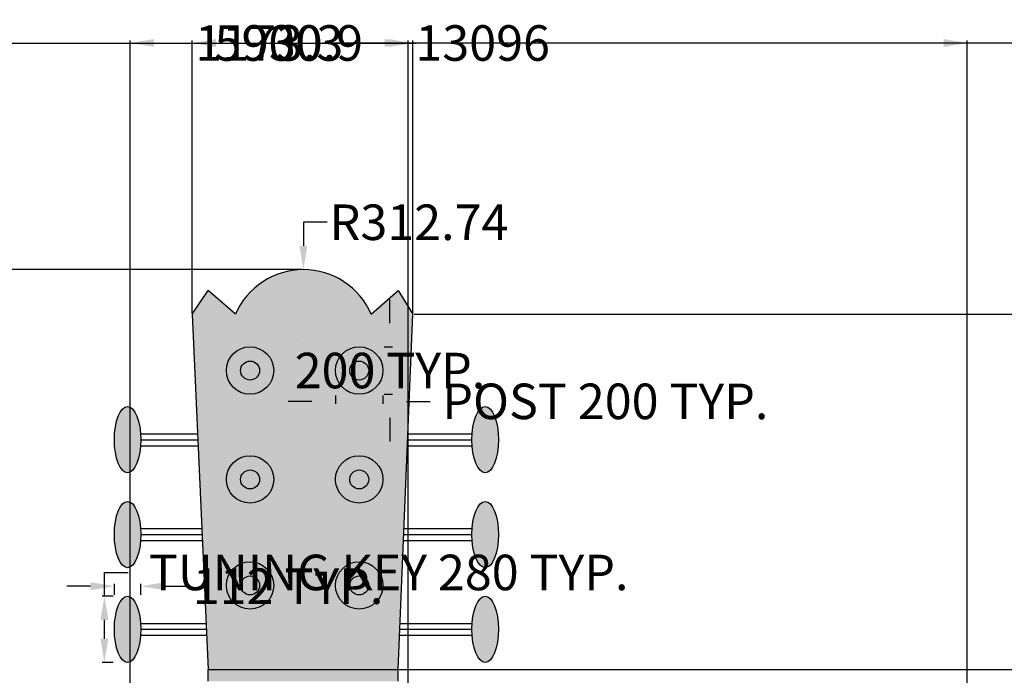
# Model space of a CAD drawing. Units: millimetres. Extents: x 11032 to 26788, y 3406 to 24505.
# Tile 77 of 78: x 16895 to 21051, y 21738 to 24505. Entities that reach past the tile are written whole.
import ezdxf

# ---------------------------------------------------------------- set-up
doc = ezdxf.new("R2010")
doc.units = ezdxf.units.MM
doc.header["$MEASUREMENT"] = 0
doc.layers.add('A-ANNO-DIMS', color=2, linetype='Continuous', lineweight=18)
doc.layers.add('A-ELEV-NECK', color=7, linetype='Continuous', lineweight=25)
doc.layers.add('A-ELEV-NECK-PATT', color=159, linetype='Continuous', lineweight=13, true_color=0x22346e)
doc.layers.add('A-ELEV-TUNE-PATT', color=251, linetype='Continuous', lineweight=13, true_color=0x636466)
doc.styles.get("Standard").update_dxf_attribs({"font": 'arial.ttf'})
doc.dimstyles.get("Standard").update_dxf_attribs({"dimtxt": 150, "dimasz": 100, "dimexe": 10, "dimexo": 5, "dimgap": 5, "dimtad": 0, "dimtih": 1, "dimtoh": 1, "dimdec": 0, "dimzin": 0, "dimdsep": 46, "dimtxsty": 'Standard', "dimcen": 0.09, "dimadec": 0, "dimazin": 0, "dimtfac": 1, "dimtdec": 0, "dimtofl": 0, "dimtmove": 0, "dimatfit": 3, "dimfxl": 1, "dimtolj": 1, "dimtzin": 0, "dimarcsym": 0})

# ---------------------------------------------------------------- blocks, each defined once
blk = doc.blocks.new('HEADSTOCK-POST')
for radius in [100, 40]:
    blk.add_circle((100, 100), radius)
blk = doc.blocks.new('TUNING-KEY-BUTTON')
blk.add_ellipse((55.9, 139.9), major_axis=(0, 139.9), ratio=0.399551)
blk = doc.blocks.new('*D26')
at = {"layer": 'A-ANNO-DIMS', "color": 0, "lineweight": -2, "transparency": 16777216}
for p, q in [((18228.1, 22919.4), (18228.1, 22884.4)), ((18428.1, 22919.4), (18428.1, 22884.4)), ((18128.1, 22894.4), (18028.1, 22894.4)), ((18528.1, 22894.4), (18628.1, 22894.4))]:
    blk.add_line(p, q, dxfattribs=at)
at = {"layer": 'A-ANNO-DIMS', "color": 0, "transparency": 16777216}
for points in [[(18128.1, 22911.1), (18128.1, 22877.8), (18228.1, 22894.4)], [(18528.1, 22911.1), (18528.1, 22877.8), (18428.1, 22894.4)]]:
    blk.add_solid(points, dxfattribs=at)
at = {"layer": 'Defpoints', "color": 0, "transparency": 16777216}
for p in [(18228.1, 22924.4), (18428.1, 22924.4), (18428.1, 22894.4)]:
    blk.add_point(p, dxfattribs=at)
at = {"layer": 'A-ANNO-DIMS', "color": 0, "transparency": 16777216, "insert": (19367.1, 22894.4), "char_height": 150, "attachment_point": 5}
blk.add_mtext('\\A1;POST 200 TYP.', dxfattribs=at)
blk = doc.blocks.new('*D27')
at = {"layer": 'A-ANNO-DIMS', "color": 0, "lineweight": -2, "transparency": 16777216}
for p, q in [((18458.1, 23224.4), (18458.1, 23324.4)), ((18433.1, 23124.4), (18468.1, 23124.4)), ((18433.1, 22924.4), (18468.1, 22924.4)), ((18458.1, 22824.4), (18458.1, 22724.4))]:
    blk.add_line(p, q, dxfattribs=at)
at = {"layer": 'A-ANNO-DIMS', "color": 0, "transparency": 16777216}
for points in [[(18441.5, 23224.4), (18474.8, 23224.4), (18458.1, 23124.4)], [(18441.5, 22824.4), (18474.8, 22824.4), (18458.1, 22924.4)]]:
    blk.add_solid(points, dxfattribs=at)
at = {"layer": 'Defpoints', "color": 0, "transparency": 16777216}
for p in [(18428.1, 23124.4), (18458.1, 23124.4), (18428.1, 22924.4)]:
    blk.add_point(p, dxfattribs=at)
at = {"layer": 'A-ANNO-DIMS', "color": 0, "transparency": 16777216, "insert": (18458.1, 23024.4), "char_height": 150, "attachment_point": 5}
blk.add_mtext('\\A1;200 TYP.', dxfattribs=at)
blk = doc.blocks.new('*D28')
at = {"layer": 'A-ANNO-DIMS', "color": 0, "lineweight": -2, "transparency": 16777216}
for p, q in [((17252.8, 22072.2), (17252.8, 22172.2)), ((17252.8, 22172.2), (17352.8, 22172.2)), ((17289.8, 22072.2), (17242.8, 22072.2)), ((17252.8, 21892.4), (17252.8, 21972.2)), ((17289.8, 21792.4), (17242.8, 21792.4))]:
    blk.add_line(p, q, dxfattribs=at)
at = {"layer": 'A-ANNO-DIMS', "color": 0, "transparency": 16777216}
for points in [[(17236.2, 21972.2), (17269.5, 21972.2), (17252.8, 22072.2)], [(17236.2, 21892.4), (17269.5, 21892.4), (17252.8, 21792.4)]]:
    blk.add_solid(points, dxfattribs=at)
at = {"layer": 'Defpoints', "color": 0, "transparency": 16777216}
for p in [(17252.8, 22072.2), (17294.8, 22072.2), (17294.8, 21792.4)]:
    blk.add_point(p, dxfattribs=at)
at = {"layer": 'A-ANNO-DIMS', "color": 0, "transparency": 16777216, "insert": (18452.5, 22172.2), "char_height": 150, "attachment_point": 5}
blk.add_mtext('\\A1;TUNING KEY 280 TYP.', dxfattribs=at)
blk = doc.blocks.new('*D29')
at = {"layer": 'A-ANNO-DIMS', "color": 0, "lineweight": -2, "transparency": 16777216}
for p, q in [((17194.8, 22114.2), (17094.8, 22114.2)), ((17294.8, 22077.2), (17294.8, 22124.2)), ((17406.6, 22077.2), (17406.6, 22124.2)), ((17506.6, 22114.2), (17606.6, 22114.2))]:
    blk.add_line(p, q, dxfattribs=at)
at = {"layer": 'A-ANNO-DIMS', "color": 0, "transparency": 16777216}
for points in [[(17194.8, 22130.9), (17194.8, 22097.5), (17294.8, 22114.2)], [(17506.6, 22130.9), (17506.6, 22097.5), (17406.6, 22114.2)]]:
    blk.add_solid(points, dxfattribs=at)
at = {"layer": 'Defpoints', "color": 0, "transparency": 16777216}
for p in [(17406.6, 22114.2), (17294.8, 22072.2), (17406.6, 22072.2)]:
    blk.add_point(p, dxfattribs=at)
at = {"layer": 'A-ANNO-DIMS', "color": 0, "transparency": 16777216, "insert": (18027.9, 22114.2), "char_height": 150, "attachment_point": 5}
blk.add_mtext('\\A1;112 TYP.', dxfattribs=at)
blk = doc.blocks.new('*D36')
at = {"layer": 'A-ANNO-DIMS', "color": 0, "lineweight": -2, "transparency": 16777216}
for p, q in [((12301.3, 17115.9), (12301.3, 24416.9)), ((12401.3, 24406.9), (18569.2, 24406.9)), ((25297.4, 24406.9), (19129.5, 24406.9)), ((25397.4, 4466.4), (25397.4, 24416.9))]:
    blk.add_line(p, q, dxfattribs=at)
at = {"layer": 'A-ANNO-DIMS', "color": 0, "transparency": 16777216}
for points in [[(12401.3, 24423.5), (12401.3, 24390.2), (12301.3, 24406.9)], [(25297.4, 24423.5), (25297.4, 24390.2), (25397.4, 24406.9)]]:
    blk.add_solid(points, dxfattribs=at)
at = {"layer": 'Defpoints', "color": 0, "transparency": 16777216}
for p in [(25397.4, 24406.9), (12301.3, 17110.9), (25397.4, 4461.4)]:
    blk.add_point(p, dxfattribs=at)
at = {"layer": 'A-ANNO-DIMS', "color": 0, "transparency": 16777216, "insert": (18849.3, 24406.9), "char_height": 150, "attachment_point": 5}
blk.add_mtext('\\A1;13096', dxfattribs=at)
blk = doc.blocks.new('*D37')
at = {"layer": 'A-ANNO-DIMS', "color": 0, "lineweight": -2, "transparency": 16777216}
for p, q in [((18087.7, 23450.4), (11334.8, 23450.4)), ((11344.8, 23350.4), (11344.8, 14037.5)), ((11344.8, 4561.4), (11344.8, 13874.3)), ((12927.7, 4461.4), (11334.8, 4461.4))]:
    blk.add_line(p, q, dxfattribs=at)
at = {"layer": 'A-ANNO-DIMS', "color": 0, "transparency": 16777216}
for points in [[(11328.1, 23350.4), (11361.4, 23350.4), (11344.8, 23450.4)], [(11328.1, 4561.4), (11361.4, 4561.4), (11344.8, 4461.4)]]:
    blk.add_solid(points, dxfattribs=at)
at = {"layer": 'Defpoints', "color": 0, "transparency": 16777216}
for p in [(11344.8, 23450.4), (18092.7, 23450.4), (12932.7, 4461.4)]:
    blk.add_point(p, dxfattribs=at)
at = {"layer": 'A-ANNO-DIMS', "color": 0, "transparency": 16777216, "insert": (11344.8, 13955.9), "char_height": 150, "attachment_point": 5}
blk.add_mtext('\\A1;18989', dxfattribs=at)
blk = doc.blocks.new('*D46')
at = {"layer": 'A-ANNO-DIMS', "color": 0, "lineweight": -2, "transparency": 16777216}
for p, q in [((18497.2, 21762.9), (26363.9, 21762.9)), ((26353.9, 21662.9), (26353.9, 20222.6)), ((26353.9, 18618.9), (26353.9, 20059.3)), ((13792.4, 18518.9), (26363.9, 18518.9))]:
    blk.add_line(p, q, dxfattribs=at)
at = {"layer": 'A-ANNO-DIMS', "color": 0, "transparency": 16777216}
for points in [[(26337.2, 21662.9), (26370.6, 21662.9), (26353.9, 21762.9)], [(26337.2, 18618.9), (26370.6, 18618.9), (26353.9, 18518.9)]]:
    blk.add_solid(points, dxfattribs=at)
at = {"layer": 'Defpoints', "color": 0, "transparency": 16777216}
for p in [(18492.2, 21762.9), (26353.9, 21762.9), (13787.4, 18518.9)]:
    blk.add_point(p, dxfattribs=at)
at = {"layer": 'A-ANNO-DIMS', "color": 0, "transparency": 16777216, "insert": (26353.9, 20140.9), "char_height": 150, "attachment_point": 5}
blk.add_mtext('\\A1;3244', dxfattribs=at)
blk = doc.blocks.new('*D47')
at = {"layer": 'A-ANNO-DIMS', "color": 0, "lineweight": -2, "transparency": 16777216}
for p, q in [((18559.6, 23262.9), (26363.9, 23262.9)), ((26353.9, 23162.9), (26353.9, 22594.5)), ((26353.9, 21862.9), (26353.9, 22431.4)), ((18497.2, 21762.9), (26363.9, 21762.9))]:
    blk.add_line(p, q, dxfattribs=at)
at = {"layer": 'A-ANNO-DIMS', "color": 0, "transparency": 16777216}
for points in [[(26337.2, 23162.9), (26370.6, 23162.9), (26353.9, 23262.9)], [(26337.2, 21862.9), (26370.6, 21862.9), (26353.9, 21762.9)]]:
    blk.add_solid(points, dxfattribs=at)
at = {"layer": 'Defpoints', "color": 0, "transparency": 16777216}
for p in [(18554.6, 23262.9), (26353.9, 23262.9), (18492.2, 21762.9)]:
    blk.add_point(p, dxfattribs=at)
at = {"layer": 'A-ANNO-DIMS', "color": 0, "transparency": 16777216, "insert": (26353.9, 22512.9), "char_height": 150, "attachment_point": 5}
blk.add_mtext('\\A1;1500', dxfattribs=at)
blk = doc.blocks.new('*D54')
at = {"layer": 'A-ANNO-DIMS', "color": 0, "lineweight": -2, "transparency": 16777216}
for p, q in [((17623.7, 23267.9), (17623.7, 24416.9)), ((17723.7, 24406.9), (17830.9, 24406.9)), ((18454.6, 24406.9), (18347.4, 24406.9)), ((18554.6, 23267.9), (18554.6, 24416.9))]:
    blk.add_line(p, q, dxfattribs=at)
at = {"layer": 'A-ANNO-DIMS', "color": 0, "transparency": 16777216}
for points in [[(17723.7, 24423.5), (17723.7, 24390.2), (17623.7, 24406.9)], [(18454.6, 24423.5), (18454.6, 24390.2), (18554.6, 24406.9)]]:
    blk.add_solid(points, dxfattribs=at)
at = {"layer": 'Defpoints', "color": 0, "transparency": 16777216}
for p in [(18554.6, 24406.9), (17623.7, 23262.9), (18554.6, 23262.9)]:
    blk.add_point(p, dxfattribs=at)
at = {"layer": 'A-ANNO-DIMS', "color": 0, "transparency": 16777216, "insert": (18089.1, 24406.9), "char_height": 150, "attachment_point": 5}
blk.add_mtext('\\A1;930.9', dxfattribs=at)
blk = doc.blocks.new('*D57')
at = {"layer": 'A-ANNO-DIMS', "color": 0, "lineweight": -2, "transparency": 16777216}
for p, q in [((14994.7, 7266.4), (14994.7, 24416.9)), ((15094.7, 24406.9), (17716, 24406.9)), ((20794.7, 24406.9), (18173.4, 24406.9)), ((20894.7, 7266.4), (20894.7, 24416.9))]:
    blk.add_line(p, q, dxfattribs=at)
at = {"layer": 'A-ANNO-DIMS', "color": 0, "transparency": 16777216}
for points in [[(15094.7, 24423.5), (15094.7, 24390.2), (14994.7, 24406.9)], [(20794.7, 24423.5), (20794.7, 24390.2), (20894.7, 24406.9)]]:
    blk.add_solid(points, dxfattribs=at)
at = {"layer": 'Defpoints', "color": 0, "transparency": 16777216}
for p in [(20894.7, 24406.9), (14994.7, 7261.4), (20894.7, 7261.4)]:
    blk.add_point(p, dxfattribs=at)
at = {"layer": 'A-ANNO-DIMS', "color": 0, "transparency": 16777216, "insert": (17944.7, 24406.9), "char_height": 150, "attachment_point": 5}
blk.add_mtext('\\A1;5900', dxfattribs=at)
blk = doc.blocks.new('*D65')
at = {"layer": 'A-ANNO-DIMS', "color": 0, "lineweight": -2, "transparency": 16777216}
for p, q in [((17362, 12566.3), (17362, 24416.9)), ((17462, 24406.9), (17639.4, 24406.9)), ((18435.4, 24406.9), (18258, 24406.9)), ((18535.4, 12566.5), (18535.4, 24416.9))]:
    blk.add_line(p, q, dxfattribs=at)
at = {"layer": 'A-ANNO-DIMS', "color": 0, "transparency": 16777216}
for points in [[(17462, 24423.5), (17462, 24390.2), (17362, 24406.9)], [(18435.4, 24423.5), (18435.4, 24390.2), (18535.4, 24406.9)]]:
    blk.add_solid(points, dxfattribs=at)
at = {"layer": 'Defpoints', "color": 0, "transparency": 16777216}
for p in [(18535.4, 24406.9), (17362, 12561.3), (18535.4, 12561.5)]:
    blk.add_point(p, dxfattribs=at)
at = {"layer": 'A-ANNO-DIMS', "color": 0, "transparency": 16777216, "insert": (17948.7, 24406.9), "char_height": 150, "attachment_point": 5}
blk.add_mtext('\\A1;1173.3', dxfattribs=at)
blk = doc.blocks.new('*D71')
at = {"layer": 'A-ANNO-DIMS', "color": 0, "lineweight": -2, "transparency": 16777216}
for p, q in [((18192.7, 23650.4), (18092.7, 23650.4)), ((18092.7, 23650.4), (18092.7, 23550.4)), ((18092.6, 23137.6), (18092.8, 23137.6)), ((18092.7, 23137.5), (18092.7, 23137.7))]:
    blk.add_line(p, q, dxfattribs=at)
at = {"layer": 'A-ANNO-DIMS', "color": 0, "transparency": 16777216}
blk.add_solid([(18076.1, 23550.4), (18109.4, 23550.4), (18092.7, 23450.4)], dxfattribs=at)
at = {"layer": 'Defpoints', "color": 0, "transparency": 16777216}
for p in [(18092.7, 23450.4), (18092.7, 23137.6)]:
    blk.add_point(p, dxfattribs=at)
at = {"layer": 'A-ANNO-DIMS', "color": 0, "transparency": 16777216, "insert": (18580.6, 23650.4), "char_height": 150, "attachment_point": 5}
blk.add_mtext('\\A1;R312.74', dxfattribs=at)

msp = doc.modelspace()

# ---------------------------------------------------------------- hatches: boundary and pattern name
at = {"layer": 'A-ELEV-NECK-PATT'}
h = msp.add_hatch(color=256, dxfattribs=at)
h.paths.add_polyline_path([(18554.563, 23262.945), (18492.19, 23362.945), (18379.27, 23262.945, 0.65407686), (17806.209, 23262.945), (17690.161, 23362.945), (17623.659, 23262.945), (17646.076, 22757.313), (18533.538, 22757.313)])
h.paths.add_polyline_path([(17967.6, 23024.435, -1), (17767.6, 23024.435, -1)], flags=16)
h.paths.add_polyline_path([(18428.148, 23024.435, -1), (18228.148, 23024.435, -1)], flags=16)
h.paths.add_polyline_path([(18531.459, 22707.313), (17648.293, 22707.313), (17663.81, 22357.313), (18516.905, 22357.313)])
h.paths.add_polyline_path([(18228.148, 22564.838, -1), (18428.148, 22564.838, -1)], flags=16)
h.paths.add_polyline_path([(17767.6, 22564.838, -1), (17967.6, 22564.838, -1)], flags=16)
h.paths.add_polyline_path([(18514.826, 22307.313), (17666.027, 22307.313), (17681.544, 21957.313), (18500.272, 21957.313)])
h.paths.add_polyline_path([(18428.148, 22117.399, -1), (18228.148, 22117.399, -1)], flags=16)
h.paths.add_polyline_path([(17967.6, 22117.399, -1), (17767.6, 22117.399, -1)], flags=16)
h.paths.add_polyline_path([(18498.193, 21907.313), (17683.761, 21907.313), (17690.161, 21762.945), (18492.19, 21762.945)])
h = msp.add_hatch(color=256, dxfattribs=at)
h.paths.add_polyline_path([(18554.563, 23262.945), (18492.19, 23362.945), (18379.27, 23262.945, 0.65407686), (17806.209, 23262.945), (17690.161, 23362.945), (17623.659, 23262.945), (17690.161, 21762.945), (18492.19, 21762.945)])
h.paths.add_polyline_path([(18428.148, 22564.838, -1), (18228.148, 22564.838, -1)], flags=16)
h.paths.add_polyline_path([(17967.6, 22564.838, -1), (17767.6, 22564.838, -1)], flags=16)
h.paths.add_polyline_path([(18368.148, 22564.838, -1), (18288.148, 22564.838, -1)], flags=0)
h.paths.add_polyline_path([(17907.6, 22564.838, -1), (17827.6, 22564.838, -1)], flags=0)
h.paths.add_polyline_path([(18228.148, 23024.435, -1), (18428.148, 23024.435, -1)], flags=16)
h.paths.add_polyline_path([(17767.6, 23024.435, -1), (17967.6, 23024.435, -1)], flags=16)
h.paths.add_polyline_path([(18288.148, 23024.435, -1), (18368.148, 23024.435, -1)], flags=0)
h.paths.add_polyline_path([(17827.6, 23024.435, -1), (17907.6, 23024.435, -1)], flags=0)
h.paths.add_polyline_path([(18428.148, 22117.399, -1), (18228.148, 22117.399, -1)], flags=16)
h.paths.add_polyline_path([(17967.6, 22117.399, -1), (17767.6, 22117.399, -1)], flags=16)
h.paths.add_polyline_path([(18368.148, 22117.399, -1), (18288.148, 22117.399, -1)], flags=0)
h.paths.add_polyline_path([(17907.6, 22117.399, -1), (17827.6, 22117.399, -1)], flags=0)
at = {"layer": 'A-ELEV-TUNE-PATT'}
h = msp.add_hatch(color=256, dxfattribs=at)
h.paths.add_polyline_path([(17967.6, 23024.435, 1), (17767.6, 23024.435, 1)])
h.paths.add_polyline_path([(17827.6, 23024.435, -1), (17907.6, 23024.435, -1)], flags=16)
h.paths.add_polyline_path([(18428.148, 23024.435, 1), (18228.148, 23024.435, 1)])
h.paths.add_polyline_path([(18288.148, 23024.435, -1), (18368.148, 23024.435, -1)], flags=16)
h.paths.add_polyline_path([(18228.148, 22564.838, 1), (18428.148, 22564.838, 1)])
h.paths.add_polyline_path([(18368.148, 22564.838, -1), (18288.148, 22564.838, -1)], flags=16)
h.paths.add_polyline_path([(17767.6, 22564.838, 1), (17967.6, 22564.838, 1)])
h.paths.add_polyline_path([(17907.6, 22564.838, -1), (17827.6, 22564.838, -1)], flags=16)
h.paths.add_polyline_path([(17967.6, 22117.399, 1), (17767.6, 22117.399, 1)])
h.paths.add_polyline_path([(17827.6, 22117.399, -1), (17907.6, 22117.399, -1)], flags=16)
h.paths.add_polyline_path([(18428.148, 22117.399, 1), (18228.148, 22117.399, 1)])
h.paths.add_polyline_path([(18288.148, 22117.399, -1), (18368.148, 22117.399, -1)], flags=16)
h = msp.add_hatch(color=256, dxfattribs=at)
h.paths.add_polyline_path([(17827.6, 22117.399, 1), (17907.6, 22117.399, 1)])
h.paths.add_polyline_path([(18368.148, 22117.399, 1), (18288.148, 22117.399, 1)])
h.paths.add_polyline_path([(18368.148, 22564.838, 1), (18288.148, 22564.838, 1)])
h.paths.add_polyline_path([(17907.6, 22564.838, 1), (17827.6, 22564.838, 1)])
h.paths.add_polyline_path([(18288.148, 23024.435, 1), (18368.148, 23024.435, 1)])
h.paths.add_polyline_path([(17907.6, 23024.435, 1), (17827.6, 23024.435, 1)])
h = msp.add_hatch(color=256, dxfattribs=at)
edge = h.paths.add_edge_path()
edge.add_ellipse((18859.87, 22732.313), major_axis=(0, 139.913), ratio=0.3995512, start_angle=114.442793, end_angle=425.557207)
edge.add_ellipse((18859.87, 22732.313), major_axis=(0, 139.913), ratio=0.3995512, start_angle=65.557207, end_angle=90)
edge.add_ellipse((18859.87, 22732.313), major_axis=(0, 139.913), ratio=0.3995512, start_angle=90, end_angle=114.442793)
edge = h.paths.add_edge_path()
edge.add_ellipse((18859.87, 22332.313), major_axis=(0, 139.913), ratio=0.3995512, start_angle=114.442793, end_angle=425.557207)
edge.add_ellipse((18859.87, 22332.313), major_axis=(0, 139.913), ratio=0.3995512, start_angle=65.557207, end_angle=90)
edge.add_ellipse((18859.87, 22332.313), major_axis=(0, 139.913), ratio=0.3995512, start_angle=90, end_angle=114.442793)
edge = h.paths.add_edge_path()
edge.add_ellipse((18859.87, 21932.313), major_axis=(0, 139.913), ratio=0.3995512, start_angle=114.442793, end_angle=425.557207)
edge.add_ellipse((18859.87, 21932.313), major_axis=(0, 139.913), ratio=0.3995512, start_angle=65.557207, end_angle=90)
edge.add_ellipse((18859.87, 21932.313), major_axis=(0, 139.913), ratio=0.3995512, start_angle=90, end_angle=114.442793)
edge = h.paths.add_edge_path()
edge.add_ellipse((17350.696, 21932.313), major_axis=(0, 139.913), ratio=0.3995512, start_angle=294.442793, end_angle=245.557207)
edge.add_ellipse((17350.696, 21932.313), major_axis=(0, 139.913), ratio=0.3995512, start_angle=245.557207, end_angle=270)
edge.add_ellipse((17350.696, 21932.313), major_axis=(0, 139.913), ratio=0.3995512, start_angle=270, end_angle=294.442793)
edge = h.paths.add_edge_path()
edge.add_ellipse((17350.696, 22332.313), major_axis=(0, 139.913), ratio=0.3995512, start_angle=270, end_angle=294.442793)
edge.add_ellipse((17350.696, 22332.313), major_axis=(0, 139.913), ratio=0.3995512, start_angle=294.442793, end_angle=245.557207)
edge.add_ellipse((17350.696, 22332.313), major_axis=(0, 139.913), ratio=0.3995512, start_angle=245.557207, end_angle=270)
h = msp.add_hatch(color=256, dxfattribs=at)
edge = h.paths.add_edge_path()
edge.add_ellipse((17350.696, 22732.313), major_axis=(0, 139.913), ratio=0.3995512, start_angle=270, end_angle=294.442793)
edge.add_ellipse((17350.696, 22732.313), major_axis=(0, 139.913), ratio=0.3995512, start_angle=294.442793, end_angle=245.557207)
edge.add_ellipse((17350.696, 22732.313), major_axis=(0, 139.913), ratio=0.3995512, start_angle=245.557207, end_angle=270)
msp.add_hatch(color=256, dxfattribs=at).paths.add_polyline_path([(18492.19, 21762.945), (17690.161, 21762.945), (17690.161, 21712.945), (18055.913, 21712.945), (18055.916, 21713.232), (18492.19, 21712.945)])

# ---------------------------------------------------------------- linework, layer by layer
at = {"layer": 'A-ELEV-NECK'}
for p, q in [((17623.659, 23262.945), (17690.161, 23362.945)), ((17806.209, 23262.945), (17690.161, 23362.945)), ((18379.27, 23262.945), (18492.19, 23362.945)), ((18492.19, 23362.945), (18554.563, 23262.945)), ((17623.659, 23262.945), (17690.161, 21762.945)), ((18492.19, 21762.945), (18554.563, 23262.945)), ((17405.699, 22757.313), (17646.076, 22757.313)), ((17406.599, 22732.313), (17647.184, 22732.313)), ((18532.498, 22732.313), (18803.967, 22732.313)), ((18533.538, 22757.313), (18804.867, 22757.313)), ((17405.699, 22707.313), (17648.293, 22707.313)), ((18531.459, 22707.313), (18804.867, 22707.313)), ((17405.699, 22357.313), (17663.81, 22357.313)), ((18516.905, 22357.313), (18804.867, 22357.313)), ((17406.599, 22332.313), (17664.918, 22332.313)), ((18515.865, 22332.313), (18803.967, 22332.313)), ((17405.699, 22307.313), (17666.027, 22307.313)), ((18514.826, 22307.313), (18804.867, 22307.313)), ((17405.699, 21957.313), (17681.544, 21957.313)), ((18500.272, 21957.313), (18804.867, 21957.313)), ((17405.699, 21907.313), (17683.761, 21907.313)), ((17406.599, 21932.313), (17682.652, 21932.313)), ((18498.193, 21907.313), (18804.867, 21907.313)), ((18499.232, 21932.313), (18803.967, 21932.313)), ((17690.161, 21762.945), (18492.19, 21762.945)), ((17690.161, 21712.945), (17690.161, 21762.945)), ((17690.161, 21762.945), (18492.19, 21762.945)), ((18056.487, 21762.945), (18081.488, 21762.945)), ((18492.19, 21712.945), (18492.19, 21762.945))]:
    msp.add_line(p, q, dxfattribs=at)
msp.add_arc((18092.739, 23137.618), 312.741, 23.624459, 156.375541, dxfattribs=at)

# ---------------------------------------------------------------- block references
for name, p in [('HEADSTOCK-POST', (17767.6, 22924.435)), ('HEADSTOCK-POST', (18228.148, 22924.435)), ('TUNING-KEY-BUTTON', (17294.793, 22592.399)), ('TUNING-KEY-BUTTON', (18803.967, 22592.399)), ('HEADSTOCK-POST', (17767.6, 22464.838)), ('HEADSTOCK-POST', (18228.148, 22464.838)), ('TUNING-KEY-BUTTON', (17294.793, 22192.399)), ('TUNING-KEY-BUTTON', (18803.967, 22192.399)), ('HEADSTOCK-POST', (17767.6, 22017.399)), ('HEADSTOCK-POST', (18228.148, 22017.399)), ('TUNING-KEY-BUTTON', (17294.793, 21792.399)), ('TUNING-KEY-BUTTON', (18803.967, 21792.399))]:
    msp.add_blockref(name, p, dxfattribs=at)

# ---------------------------------------------------------------- dimensions: what is measured, and where the dimension line sits
at = {"layer": 'A-ANNO-DIMS'}
for base, p1, p2, override, picture, middle in [((25397.404, 24406.858), (12301.265, 17110.885), (25397.404, 4461.399), {"dimdec": 0, "dimlfac": 1, "dimrnd": 0, "dimzin": 0, "dimdsep": 46, "dimlunit": 2}, '*D36', (18849.334, 24406.858)), ((20894.704, 24406.858), (14994.704, 7261.399), (20894.704, 7261.399), {"dimdec": 0, "dimlfac": 1, "dimrnd": 0, "dimzin": 0, "dimdsep": 46, "dimlunit": 2}, '*D57', (17944.704, 24406.858)), ((18535.366, 24406.858), (17362.033, 12561.3), (18535.366, 12561.507), {"dimdec": 1, "dimlfac": 1, "dimrnd": 0, "dimzin": 0, "dimdsep": 46, "dimlunit": 2}, '*D65', (17948.7, 24406.858)), ((18554.563, 24406.858), (17623.659, 23262.945), (18554.563, 23262.945), {"dimdec": 1, "dimlfac": 1, "dimrnd": 0, "dimzin": 0, "dimdsep": 46, "dimlunit": 2}, '*D54', (18089.111, 24406.858))]:
    dim = msp.add_linear_dim(base=base, p1=p1, p2=p2, dimstyle='Standard', override=override, dxfattribs=at)
    dim.commit()
    dim.dimension.update_dxf_attribs({"geometry": picture, "text_midpoint": middle})
dim = msp.add_radius_dim(center=(18092.739, 23137.618), mpoint=(18092.739, 23450.358), dimstyle='Standard', override={"dimdec": 2, "dimlfac": 1, "dimrnd": 0, "dimzin": 0, "dimdsep": 46, "dimlunit": 2}, dxfattribs=at)
dim.commit()
dim.dimension.update_dxf_attribs({"geometry": '*D71', "text_midpoint": (18580.566, 23650.358)})
for base, p1, p2, picture, middle in [((11344.765, 23450.358), (12932.665, 4461.399), (18092.739, 23450.358), '*D37', (11344.765, 13955.879)), ((26353.904, 23262.945), (18492.19, 21762.945), (18554.563, 23262.945), '*D47', (26353.904, 22512.945)), ((26353.904, 21762.945), (13787.367, 18518.925), (18492.19, 21762.945), '*D46', (26353.904, 20140.935))]:
    dim = msp.add_linear_dim(base=base, p1=p1, p2=p2, angle=90, dimstyle='Standard', override={"dimdec": 0, "dimlfac": 1, "dimrnd": 0, "dimzin": 0, "dimdsep": 46, "dimlunit": 2}, dxfattribs=at)
    dim.commit()
    dim.dimension.update_dxf_attribs({"geometry": picture, "text_midpoint": middle})
for base, p1, p2, text, picture, middle in [((18458.148, 23124.435), (18428.148, 22924.435), (18428.148, 23124.435), '<> TYP.', '*D27', (18458.148, 23024.435)), ((17252.819, 22072.226), (17294.793, 21792.399), (17294.793, 22072.226), 'TUNING KEY <> TYP.', '*D28', (18452.533, 22172.226))]:
    dim = msp.add_linear_dim(base=base, p1=p1, p2=p2, angle=90, text=text, dimstyle='Standard', override={"dimdec": 0, "dimlfac": 1, "dimrnd": 0, "dimzin": 0, "dimdsep": 46, "dimlunit": 2}, dxfattribs=at)
    dim.commit()
    dim.dimension.update_dxf_attribs({"geometry": picture, "text_midpoint": middle})
for base, p1, p2, text, picture, middle in [((18428.148, 22894.435), (18228.148, 22924.435), (18428.148, 22924.435), 'POST <> TYP.', '*D26', (19367.135, 22894.435)), ((17406.599, 22114.2), (17294.793, 22072.226), (17406.599, 22072.226), '<> TYP.', '*D29', (18027.884, 22114.2))]:
    dim = msp.add_linear_dim(base=base, p1=p1, p2=p2, text=text, dimstyle='Standard', override={"dimdec": 0, "dimlfac": 1, "dimrnd": 0, "dimzin": 0, "dimdsep": 46, "dimlunit": 2}, dxfattribs=at)
    dim.commit()
    dim.dimension.update_dxf_attribs({"geometry": picture, "text_midpoint": middle})

doc.saveas('drawing.dxf')
